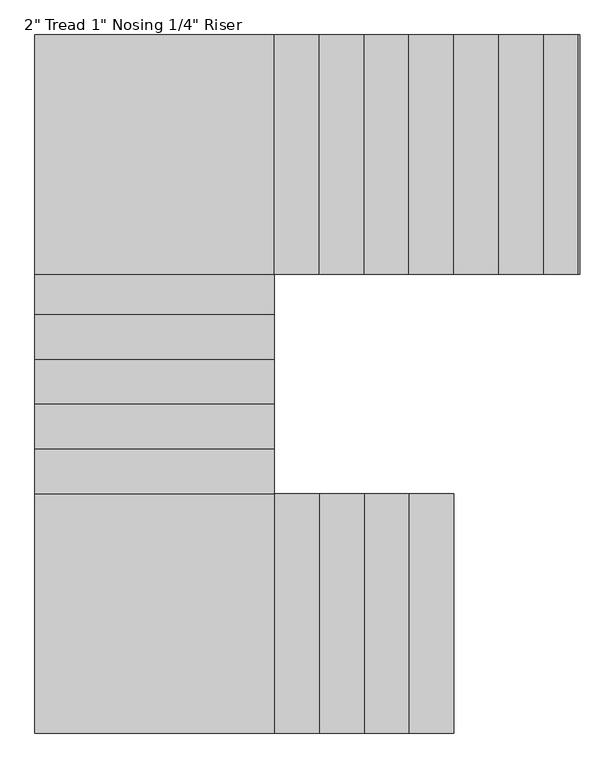
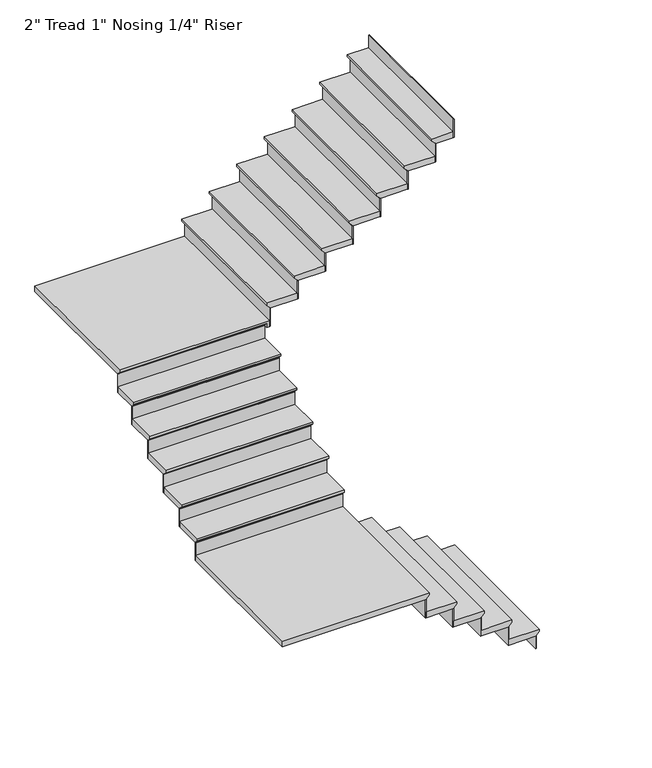
"""IFC4 building model written with IfcOpenShell, lengths in millimetres: stair flight geometry."""

from ifc_helpers import new_model, si_unit, origin, place, context, project, spatial, faceted_brep, source, transform, mapped, element, save


def stair_flight_0ad16ec4(model_context):
    return source(origin(), model_context, "Body", "Brep", [
        faceted_brep([(-2683.1105391, -1521.8373761, 141.3710526), (-2683.1105391, -1521.8373761, 160.4210526), (-2683.1105391, -2741.0373761, 160.4210526), (-2683.1105391, -2741.0373761, 141.3710526), (-2708.5105391, -1521.8373761, 115.9710526), (-2708.5105391, -2741.0373761, 115.9710526), (-2937.1105391, -1521.8373761, 160.4210526), (-2937.1105391, -2741.0373761, 160.4210526), (-2708.5105391, -2741.0373761, 109.6210526), (-2937.1105391, -2741.0373761, 109.6210526), (-2937.1105391, -1521.8373761, 109.6210526), (-2708.5105391, -1521.8373761, 109.6210526)], [[[0, 1, 2, 3]], [[4, 0, 3, 5]], [[2, 1, 6, 7]], [[8, 9, 10, 11]], [[2, 7, 9, 8, 5, 3]], [[8, 11, 4, 5]], [[6, 1, 0, 4, 11, 10]], [[7, 6, 10, 9]]]),
        faceted_brep([(-2708.5105391, -1521.8373761, 109.6210526), (-2708.5105391, -1521.8373761, 0.0), (-2714.8605391, -1521.8373761, 0.0), (-2714.8605391, -1521.8373761, 109.6210526), (-2708.5105391, -2741.0373761, 109.6210526), (-2714.8605391, -2741.0373761, 109.6210526), (-2714.8605391, -2741.0373761, 0.0), (-2708.5105391, -2741.0373761, 0.0)], [[[0, 1, 2, 3]], [[4, 5, 6, 7]], [[1, 0, 4, 7]], [[2, 1, 7, 6]], [[3, 2, 6, 5]], [[0, 3, 5, 4]]]),
        faceted_brep([(-2937.1105391, -1521.8373761, 270.0421053), (-2937.1105391, -1521.8373761, 109.6210526), (-2943.4605391, -1521.8373761, 109.6210526), (-2943.4605391, -1521.8373761, 270.0421053), (-2937.1105391, -2741.0373761, 270.0421053), (-2943.4605391, -2741.0373761, 270.0421053), (-2943.4605391, -2741.0373761, 109.6210526), (-2937.1105391, -2741.0373761, 109.6210526)], [[[0, 1, 2, 3]], [[4, 5, 6, 7]], [[1, 0, 4, 7]], [[2, 1, 7, 6]], [[3, 2, 6, 5]], [[0, 3, 5, 4]]]),
        faceted_brep([(-2911.7105391, -2741.0373761, 320.8421053), (-2911.7105391, -1521.8373761, 320.8421053), (-3165.7105391, -1521.8373761, 320.8421053), (-3165.7105391, -2741.0373761, 320.8421053), (-2937.1105391, -2741.0373761, 270.0421053), (-3165.7105391, -2741.0373761, 270.0421053), (-3165.7105391, -1521.8373761, 270.0421053), (-2937.1105391, -1521.8373761, 270.0421053), (-2937.1105391, -2741.0373761, 276.3921053), (-2911.7105391, -2741.0373761, 301.7921053), (-2937.1105391, -1521.8373761, 276.3921053), (-2911.7105391, -1521.8373761, 301.7921053)], [[[0, 1, 2, 3]], [[4, 5, 6, 7]], [[0, 3, 5, 4, 8, 9]], [[4, 7, 10, 8]], [[2, 1, 11, 10, 7, 6]], [[3, 2, 6, 5]], [[11, 1, 0, 9]], [[10, 11, 9, 8]]]),
        faceted_brep([(-3165.7105391, -1521.8373761, 430.4631579), (-3165.7105391, -1521.8373761, 270.0421053), (-3172.0605391, -1521.8373761, 270.0421053), (-3172.0605391, -1521.8373761, 430.4631579), (-3165.7105391, -2741.0373761, 430.4631579), (-3172.0605391, -2741.0373761, 430.4631579), (-3172.0605391, -2741.0373761, 270.0421053), (-3165.7105391, -2741.0373761, 270.0421053)], [[[0, 1, 2, 3]], [[4, 5, 6, 7]], [[1, 0, 4, 7]], [[2, 1, 7, 6]], [[3, 2, 6, 5]], [[0, 3, 5, 4]]]),
        faceted_brep([(-3140.3105391, -2741.0373761, 481.2631579), (-3140.3105391, -1521.8373761, 481.2631579), (-3394.3105391, -1521.8373761, 481.2631579), (-3394.3105391, -2741.0373761, 481.2631579), (-3165.7105391, -2741.0373761, 430.4631579), (-3394.3105391, -2741.0373761, 430.4631579), (-3394.3105391, -1521.8373761, 430.4631579), (-3165.7105391, -1521.8373761, 430.4631579), (-3165.7105391, -2741.0373761, 436.8131579), (-3140.3105391, -2741.0373761, 462.2131579), (-3165.7105391, -1521.8373761, 436.8131579), (-3140.3105391, -1521.8373761, 462.2131579)], [[[0, 1, 2, 3]], [[4, 5, 6, 7]], [[0, 3, 5, 4, 8, 9]], [[4, 7, 10, 8]], [[2, 1, 11, 10, 7, 6]], [[3, 2, 6, 5]], [[11, 1, 0, 9]], [[10, 11, 9, 8]]]),
        faceted_brep([(-3394.3105391, -1521.8373761, 590.8842105), (-3394.3105391, -1521.8373761, 430.4631579), (-3400.6605391, -1521.8373761, 430.4631579), (-3400.6605391, -1521.8373761, 590.8842105), (-3394.3105391, -2741.0373761, 590.8842105), (-3400.6605391, -2741.0373761, 590.8842105), (-3400.6605391, -2741.0373761, 430.4631579), (-3394.3105391, -2741.0373761, 430.4631579)], [[[0, 1, 2, 3]], [[4, 5, 6, 7]], [[1, 0, 4, 7]], [[2, 1, 7, 6]], [[3, 2, 6, 5]], [[0, 3, 5, 4]]]),
        faceted_brep([(-3368.9105391, -2741.0373761, 641.6842105), (-3368.9105391, -1521.8373761, 641.6842105), (-3622.9105391, -1521.8373761, 641.6842105), (-3622.9105391, -2741.0373761, 641.6842105), (-3394.3105391, -2741.0373761, 590.8842105), (-3622.9105391, -2741.0373761, 590.8842105), (-3622.9105391, -1521.8373761, 590.8842105), (-3394.3105391, -1521.8373761, 590.8842105), (-3394.3105391, -2741.0373761, 597.2342105), (-3368.9105391, -2741.0373761, 622.6342105), (-3394.3105391, -1521.8373761, 597.2342105), (-3368.9105391, -1521.8373761, 622.6342105)], [[[0, 1, 2, 3]], [[4, 5, 6, 7]], [[0, 3, 5, 4, 8, 9]], [[4, 7, 10, 8]], [[2, 1, 11, 10, 7, 6]], [[3, 2, 6, 5]], [[11, 1, 0, 9]], [[10, 11, 9, 8]]]),
        faceted_brep([(-3622.9105391, -1521.8373761, 751.3052632), (-3622.9105391, -1521.8373761, 590.8842105), (-3629.2605391, -1521.8373761, 590.8842105), (-3629.2605391, -1521.8373761, 751.3052632), (-3622.9105391, -2741.0373761, 751.3052632), (-3629.2605391, -2741.0373761, 751.3052632), (-3629.2605391, -2741.0373761, 590.8842105), (-3622.9105391, -2741.0373761, 590.8842105)], [[[0, 1, 2, 3]], [[4, 5, 6, 7]], [[1, 0, 4, 7]], [[2, 1, 7, 6]], [[3, 2, 6, 5]], [[0, 3, 5, 4]]]),
        faceted_brep([(-4816.7105391, -1496.4373761, 802.1052632), (-4816.7105391, -2741.0373761, 802.1052632), (-3597.5105391, -2741.0373761, 802.1052632), (-3597.5105391, -1496.4373761, 802.1052632), (-4816.7105391, -2741.0373761, 751.3052632), (-4816.7105391, -1496.4373761, 751.3052632), (-3597.5105391, -1496.4373761, 751.3052632), (-3597.5105391, -1521.8373761, 751.3052632), (-3622.9105391, -1521.8373761, 751.3052632), (-3622.9105391, -2741.0373761, 751.3052632), (-3622.9105391, -2741.0373761, 757.6552632), (-3597.5105391, -2741.0373761, 783.0552632), (-3622.9105391, -1521.8373761, 757.6552632), (-3597.5105391, -1521.8373761, 783.0552632)], [[[0, 1, 2, 3]], [[4, 5, 6, 7, 8, 9]], [[1, 0, 5, 4]], [[2, 1, 4, 9, 10, 11]], [[9, 8, 12, 10]], [[8, 7, 13, 12]], [[3, 2, 11, 13, 7, 6]], [[0, 3, 6, 5]], [[11, 10, 12, 13]]]),
        faceted_brep([(-3597.5105391, -1496.4373761, 911.7263158), (-3597.5105391, -1496.4373761, 751.3052632), (-3597.5105391, -1490.0873761, 751.3052632), (-3597.5105391, -1490.0873761, 911.7263158), (-4816.7105391, -1496.4373761, 911.7263158), (-4816.7105391, -1490.0873761, 911.7263158), (-4816.7105391, -1490.0873761, 751.3052632), (-4816.7105391, -1496.4373761, 751.3052632)], [[[0, 1, 2, 3]], [[4, 5, 6, 7]], [[1, 0, 4, 7]], [[2, 1, 7, 6]], [[3, 2, 6, 5]], [[0, 3, 5, 4]]]),
        faceted_brep([(-4816.7105391, -1521.8373761, 962.5263158), (-3597.5105391, -1521.8373761, 962.5263158), (-3597.5105391, -1267.8373761, 962.5263158), (-4816.7105391, -1267.8373761, 962.5263158), (-4816.7105391, -1496.4373761, 911.7263158), (-4816.7105391, -1267.8373761, 911.7263158), (-3597.5105391, -1267.8373761, 911.7263158), (-3597.5105391, -1496.4373761, 911.7263158), (-4816.7105391, -1496.4373761, 918.0763158), (-4816.7105391, -1521.8373761, 943.4763158), (-3597.5105391, -1496.4373761, 918.0763158), (-3597.5105391, -1521.8373761, 943.4763158)], [[[0, 1, 2, 3]], [[4, 5, 6, 7]], [[0, 3, 5, 4, 8, 9]], [[4, 7, 10, 8]], [[2, 1, 11, 10, 7, 6]], [[3, 2, 6, 5]], [[11, 1, 0, 9]], [[10, 11, 9, 8]]]),
        faceted_brep([(-3597.5105391, -1267.8373761, 1072.1473684), (-3597.5105391, -1267.8373761, 911.7263158), (-3597.5105391, -1261.4873761, 911.7263158), (-3597.5105391, -1261.4873761, 1072.1473684), (-4816.7105391, -1267.8373761, 1072.1473684), (-4816.7105391, -1261.4873761, 1072.1473684), (-4816.7105391, -1261.4873761, 911.7263158), (-4816.7105391, -1267.8373761, 911.7263158)], [[[0, 1, 2, 3]], [[4, 5, 6, 7]], [[1, 0, 4, 7]], [[2, 1, 7, 6]], [[3, 2, 6, 5]], [[0, 3, 5, 4]]]),
        faceted_brep([(-4816.7105391, -1293.2373761, 1122.9473684), (-3597.5105391, -1293.2373761, 1122.9473684), (-3597.5105391, -1039.2373761, 1122.9473684), (-4816.7105391, -1039.2373761, 1122.9473684), (-4816.7105391, -1267.8373761, 1072.1473684), (-4816.7105391, -1039.2373761, 1072.1473684), (-3597.5105391, -1039.2373761, 1072.1473684), (-3597.5105391, -1267.8373761, 1072.1473684), (-4816.7105391, -1267.8373761, 1078.4973684), (-4816.7105391, -1293.2373761, 1103.8973684), (-3597.5105391, -1267.8373761, 1078.4973684), (-3597.5105391, -1293.2373761, 1103.8973684)], [[[0, 1, 2, 3]], [[4, 5, 6, 7]], [[0, 3, 5, 4, 8, 9]], [[4, 7, 10, 8]], [[2, 1, 11, 10, 7, 6]], [[3, 2, 6, 5]], [[11, 1, 0, 9]], [[10, 11, 9, 8]]]),
        faceted_brep([(-3597.5105391, -1039.2373761, 1232.5684211), (-3597.5105391, -1039.2373761, 1072.1473684), (-3597.5105391, -1032.8873761, 1072.1473684), (-3597.5105391, -1032.8873761, 1232.5684211), (-4816.7105391, -1039.2373761, 1232.5684211), (-4816.7105391, -1032.8873761, 1232.5684211), (-4816.7105391, -1032.8873761, 1072.1473684), (-4816.7105391, -1039.2373761, 1072.1473684)], [[[0, 1, 2, 3]], [[4, 5, 6, 7]], [[1, 0, 4, 7]], [[2, 1, 7, 6]], [[3, 2, 6, 5]], [[0, 3, 5, 4]]]),
        faceted_brep([(-4816.7105391, -1064.6373761, 1283.3684211), (-3597.5105391, -1064.6373761, 1283.3684211), (-3597.5105391, -810.6373761, 1283.3684211), (-4816.7105391, -810.6373761, 1283.3684211), (-4816.7105391, -1039.2373761, 1232.5684211), (-4816.7105391, -810.6373761, 1232.5684211), (-3597.5105391, -810.6373761, 1232.5684211), (-3597.5105391, -1039.2373761, 1232.5684211), (-4816.7105391, -1039.2373761, 1238.9184211), (-4816.7105391, -1064.6373761, 1264.3184211), (-3597.5105391, -1039.2373761, 1238.9184211), (-3597.5105391, -1064.6373761, 1264.3184211)], [[[0, 1, 2, 3]], [[4, 5, 6, 7]], [[0, 3, 5, 4, 8, 9]], [[4, 7, 10, 8]], [[2, 1, 11, 10, 7, 6]], [[3, 2, 6, 5]], [[11, 1, 0, 9]], [[10, 11, 9, 8]]]),
        faceted_brep([(-3597.5105391, -810.6373761, 1392.9894737), (-3597.5105391, -810.6373761, 1232.5684211), (-3597.5105391, -804.2873761, 1232.5684211), (-3597.5105391, -804.2873761, 1392.9894737), (-4816.7105391, -810.6373761, 1392.9894737), (-4816.7105391, -804.2873761, 1392.9894737), (-4816.7105391, -804.2873761, 1232.5684211), (-4816.7105391, -810.6373761, 1232.5684211)], [[[0, 1, 2, 3]], [[4, 5, 6, 7]], [[1, 0, 4, 7]], [[2, 1, 7, 6]], [[3, 2, 6, 5]], [[0, 3, 5, 4]]]),
        faceted_brep([(-4816.7105391, -836.0373761, 1443.7894737), (-3597.5105391, -836.0373761, 1443.7894737), (-3597.5105391, -582.0373761, 1443.7894737), (-4816.7105391, -582.0373761, 1443.7894737), (-4816.7105391, -810.6373761, 1392.9894737), (-4816.7105391, -582.0373761, 1392.9894737), (-3597.5105391, -582.0373761, 1392.9894737), (-3597.5105391, -810.6373761, 1392.9894737), (-4816.7105391, -810.6373761, 1399.3394737), (-4816.7105391, -836.0373761, 1424.7394737), (-3597.5105391, -810.6373761, 1399.3394737), (-3597.5105391, -836.0373761, 1424.7394737)], [[[0, 1, 2, 3]], [[4, 5, 6, 7]], [[0, 3, 5, 4, 8, 9]], [[4, 7, 10, 8]], [[2, 1, 11, 10, 7, 6]], [[3, 2, 6, 5]], [[11, 1, 0, 9]], [[10, 11, 9, 8]]]),
        faceted_brep([(-3597.5105391, -582.0373761, 1553.4105263), (-3597.5105391, -582.0373761, 1392.9894737), (-3597.5105391, -575.6873761, 1392.9894737), (-3597.5105391, -575.6873761, 1553.4105263), (-4816.7105391, -582.0373761, 1553.4105263), (-4816.7105391, -575.6873761, 1553.4105263), (-4816.7105391, -575.6873761, 1392.9894737), (-4816.7105391, -582.0373761, 1392.9894737)], [[[0, 1, 2, 3]], [[4, 5, 6, 7]], [[1, 0, 4, 7]], [[2, 1, 7, 6]], [[3, 2, 6, 5]], [[0, 3, 5, 4]]]),
        faceted_brep([(-4816.7105391, -607.4373761, 1604.2105263), (-3597.5105391, -607.4373761, 1604.2105263), (-3597.5105391, -378.8373761, 1604.2105263), (-4816.7105391, -378.8373761, 1604.2105263), (-4816.7105391, -582.0373761, 1553.4105263), (-4816.7105391, -378.8373761, 1553.4105263), (-3597.5105391, -378.8373761, 1553.4105263), (-3597.5105391, -582.0373761, 1553.4105263), (-4816.7105391, -582.0373761, 1559.7605263), (-4816.7105391, -607.4373761, 1585.1605263), (-3597.5105391, -582.0373761, 1559.7605263), (-3597.5105391, -607.4373761, 1585.1605263)], [[[0, 1, 2, 3]], [[4, 5, 6, 7]], [[0, 3, 5, 4, 8, 9]], [[4, 7, 10, 8]], [[2, 1, 11, 10, 7, 6]], [[3, 2, 6, 5]], [[11, 1, 0, 9]], [[10, 11, 9, 8]]]),
        faceted_brep([(-3597.5105391, -378.8373761, 1713.8315789), (-3597.5105391, -378.8373761, 1553.4105263), (-3597.5105391, -372.4873761, 1553.4105263), (-3597.5105391, -372.4873761, 1713.8315789), (-4816.7105391, -378.8373761, 1713.8315789), (-4816.7105391, -372.4873761, 1713.8315789), (-4816.7105391, -372.4873761, 1553.4105263), (-4816.7105391, -378.8373761, 1553.4105263)], [[[0, 1, 2, 3]], [[4, 5, 6, 7]], [[1, 0, 4, 7]], [[2, 1, 7, 6]], [[3, 2, 6, 5]], [[0, 3, 5, 4]]]),
        faceted_brep([(-3572.1105391, 814.9626239, 1764.6315789), (-4816.7105391, 814.9626239, 1764.6315789), (-4816.7105391, -404.2373761, 1764.6315789), (-3572.1105391, -404.2373761, 1764.6315789), (-4816.7105391, 814.9626239, 1713.8315789), (-3572.1105391, 814.9626239, 1713.8315789), (-3572.1105391, -404.2373761, 1713.8315789), (-3597.5105391, -404.2373761, 1713.8315789), (-3597.5105391, -378.8373761, 1713.8315789), (-4816.7105391, -378.8373761, 1713.8315789), (-4816.7105391, -378.8373761, 1720.1815789), (-4816.7105391, -404.2373761, 1745.5815789), (-3597.5105391, -378.8373761, 1720.1815789), (-3597.5105391, -404.2373761, 1745.5815789)], [[[0, 1, 2, 3]], [[4, 5, 6, 7, 8, 9]], [[1, 0, 5, 4]], [[2, 1, 4, 9, 10, 11]], [[9, 8, 12, 10]], [[8, 7, 13, 12]], [[3, 2, 11, 13, 7, 6]], [[0, 3, 6, 5]], [[11, 10, 12, 13]]]),
        faceted_brep([(-3572.1105391, -404.2373761, 1874.2526316), (-3572.1105391, -404.2373761, 1713.8315789), (-3565.7605391, -404.2373761, 1713.8315789), (-3565.7605391, -404.2373761, 1874.2526316), (-3572.1105391, 814.9626239, 1874.2526316), (-3565.7605391, 814.9626239, 1874.2526316), (-3565.7605391, 814.9626239, 1713.8315789), (-3572.1105391, 814.9626239, 1713.8315789)], [[[0, 1, 2, 3]], [[4, 5, 6, 7]], [[1, 0, 4, 7]], [[2, 1, 7, 6]], [[3, 2, 6, 5]], [[0, 3, 5, 4]]]),
        faceted_brep([(-3597.5105391, 814.9626239, 1925.0526316), (-3597.5105391, -404.2373761, 1925.0526316), (-3343.5105391, -404.2373761, 1925.0526316), (-3343.5105391, 814.9626239, 1925.0526316), (-3572.1105391, 814.9626239, 1874.2526316), (-3343.5105391, 814.9626239, 1874.2526316), (-3343.5105391, -404.2373761, 1874.2526316), (-3572.1105391, -404.2373761, 1874.2526316), (-3572.1105391, 814.9626239, 1880.6026316), (-3597.5105391, 814.9626239, 1906.0026316), (-3572.1105391, -404.2373761, 1880.6026316), (-3597.5105391, -404.2373761, 1906.0026316)], [[[0, 1, 2, 3]], [[4, 5, 6, 7]], [[0, 3, 5, 4, 8, 9]], [[4, 7, 10, 8]], [[2, 1, 11, 10, 7, 6]], [[3, 2, 6, 5]], [[11, 1, 0, 9]], [[10, 11, 9, 8]]]),
        faceted_brep([(-3343.5105391, -404.2373761, 2034.6736842), (-3343.5105391, -404.2373761, 1874.2526316), (-3337.1605391, -404.2373761, 1874.2526316), (-3337.1605391, -404.2373761, 2034.6736842), (-3343.5105391, 814.9626239, 2034.6736842), (-3337.1605391, 814.9626239, 2034.6736842), (-3337.1605391, 814.9626239, 1874.2526316), (-3343.5105391, 814.9626239, 1874.2526316)], [[[0, 1, 2, 3]], [[4, 5, 6, 7]], [[1, 0, 4, 7]], [[2, 1, 7, 6]], [[3, 2, 6, 5]], [[0, 3, 5, 4]]]),
        faceted_brep([(-3368.9105391, 814.9626239, 2085.4736842), (-3368.9105391, -404.2373761, 2085.4736842), (-3114.9105391, -404.2373761, 2085.4736842), (-3114.9105391, 814.9626239, 2085.4736842), (-3343.5105391, 814.9626239, 2034.6736842), (-3114.9105391, 814.9626239, 2034.6736842), (-3114.9105391, -404.2373761, 2034.6736842), (-3343.5105391, -404.2373761, 2034.6736842), (-3343.5105391, 814.9626239, 2041.0236842), (-3368.9105391, 814.9626239, 2066.4236842), (-3343.5105391, -404.2373761, 2041.0236842), (-3368.9105391, -404.2373761, 2066.4236842)], [[[0, 1, 2, 3]], [[4, 5, 6, 7]], [[0, 3, 5, 4, 8, 9]], [[4, 7, 10, 8]], [[2, 1, 11, 10, 7, 6]], [[3, 2, 6, 5]], [[11, 1, 0, 9]], [[10, 11, 9, 8]]]),
        faceted_brep([(-3114.9105391, -404.2373761, 2195.0947368), (-3114.9105391, -404.2373761, 2034.6736842), (-3108.5605391, -404.2373761, 2034.6736842), (-3108.5605391, -404.2373761, 2195.0947368), (-3114.9105391, 814.9626239, 2195.0947368), (-3108.5605391, 814.9626239, 2195.0947368), (-3108.5605391, 814.9626239, 2034.6736842), (-3114.9105391, 814.9626239, 2034.6736842)], [[[0, 1, 2, 3]], [[4, 5, 6, 7]], [[1, 0, 4, 7]], [[2, 1, 7, 6]], [[3, 2, 6, 5]], [[0, 3, 5, 4]]]),
        faceted_brep([(-3140.3105391, 814.9626239, 2245.8947368), (-3140.3105391, -404.2373761, 2245.8947368), (-2886.3105391, -404.2373761, 2245.8947368), (-2886.3105391, 814.9626239, 2245.8947368), (-3114.9105391, 814.9626239, 2195.0947368), (-2886.3105391, 814.9626239, 2195.0947368), (-2886.3105391, -404.2373761, 2195.0947368), (-3114.9105391, -404.2373761, 2195.0947368), (-3114.9105391, 814.9626239, 2201.4447368), (-3140.3105391, 814.9626239, 2226.8447368), (-3114.9105391, -404.2373761, 2201.4447368), (-3140.3105391, -404.2373761, 2226.8447368)], [[[0, 1, 2, 3]], [[4, 5, 6, 7]], [[0, 3, 5, 4, 8, 9]], [[4, 7, 10, 8]], [[2, 1, 11, 10, 7, 6]], [[3, 2, 6, 5]], [[11, 1, 0, 9]], [[10, 11, 9, 8]]]),
        faceted_brep([(-2886.3105391, -404.2373761, 2355.5157895), (-2886.3105391, -404.2373761, 2195.0947368), (-2879.9605391, -404.2373761, 2195.0947368), (-2879.9605391, -404.2373761, 2355.5157895), (-2886.3105391, 814.9626239, 2355.5157895), (-2879.9605391, 814.9626239, 2355.5157895), (-2879.9605391, 814.9626239, 2195.0947368), (-2886.3105391, 814.9626239, 2195.0947368)], [[[0, 1, 2, 3]], [[4, 5, 6, 7]], [[1, 0, 4, 7]], [[2, 1, 7, 6]], [[3, 2, 6, 5]], [[0, 3, 5, 4]]]),
        faceted_brep([(-2911.7105391, 814.9626239, 2406.3157895), (-2911.7105391, -404.2373761, 2406.3157895), (-2657.7105391, -404.2373761, 2406.3157895), (-2657.7105391, 814.9626239, 2406.3157895), (-2886.3105391, 814.9626239, 2355.5157895), (-2657.7105391, 814.9626239, 2355.5157895), (-2657.7105391, -404.2373761, 2355.5157895), (-2886.3105391, -404.2373761, 2355.5157895), (-2886.3105391, 814.9626239, 2361.8657895), (-2911.7105391, 814.9626239, 2387.2657895), (-2886.3105391, -404.2373761, 2361.8657895), (-2911.7105391, -404.2373761, 2387.2657895)], [[[0, 1, 2, 3]], [[4, 5, 6, 7]], [[0, 3, 5, 4, 8, 9]], [[4, 7, 10, 8]], [[2, 1, 11, 10, 7, 6]], [[3, 2, 6, 5]], [[11, 1, 0, 9]], [[10, 11, 9, 8]]]),
        faceted_brep([(-2657.7105391, -404.2373761, 2515.9368421), (-2657.7105391, -404.2373761, 2355.5157895), (-2651.3605391, -404.2373761, 2355.5157895), (-2651.3605391, -404.2373761, 2515.9368421), (-2657.7105391, 814.9626239, 2515.9368421), (-2651.3605391, 814.9626239, 2515.9368421), (-2651.3605391, 814.9626239, 2355.5157895), (-2657.7105391, 814.9626239, 2355.5157895)], [[[0, 1, 2, 3]], [[4, 5, 6, 7]], [[1, 0, 4, 7]], [[2, 1, 7, 6]], [[3, 2, 6, 5]], [[0, 3, 5, 4]]]),
        faceted_brep([(-2683.1105391, 814.9626239, 2566.7368421), (-2683.1105391, -404.2373761, 2566.7368421), (-2429.1105391, -404.2373761, 2566.7368421), (-2429.1105391, 814.9626239, 2566.7368421), (-2657.7105391, 814.9626239, 2515.9368421), (-2429.1105391, 814.9626239, 2515.9368421), (-2429.1105391, -404.2373761, 2515.9368421), (-2657.7105391, -404.2373761, 2515.9368421), (-2657.7105391, 814.9626239, 2522.2868421), (-2683.1105391, 814.9626239, 2547.6868421), (-2657.7105391, -404.2373761, 2522.2868421), (-2683.1105391, -404.2373761, 2547.6868421)], [[[0, 1, 2, 3]], [[4, 5, 6, 7]], [[0, 3, 5, 4, 8, 9]], [[4, 7, 10, 8]], [[2, 1, 11, 10, 7, 6]], [[3, 2, 6, 5]], [[11, 1, 0, 9]], [[10, 11, 9, 8]]]),
        faceted_brep([(-2429.1105391, -404.2373761, 2676.3578947), (-2429.1105391, -404.2373761, 2515.9368421), (-2422.7605391, -404.2373761, 2515.9368421), (-2422.7605391, -404.2373761, 2676.3578947), (-2429.1105391, 814.9626239, 2676.3578947), (-2422.7605391, 814.9626239, 2676.3578947), (-2422.7605391, 814.9626239, 2515.9368421), (-2429.1105391, 814.9626239, 2515.9368421)], [[[0, 1, 2, 3]], [[4, 5, 6, 7]], [[1, 0, 4, 7]], [[2, 1, 7, 6]], [[3, 2, 6, 5]], [[0, 3, 5, 4]]]),
        faceted_brep([(-2454.5105391, 814.9626239, 2727.1578947), (-2454.5105391, -404.2373761, 2727.1578947), (-2200.5105391, -404.2373761, 2727.1578947), (-2200.5105391, 814.9626239, 2727.1578947), (-2429.1105391, 814.9626239, 2676.3578947), (-2200.5105391, 814.9626239, 2676.3578947), (-2200.5105391, -404.2373761, 2676.3578947), (-2429.1105391, -404.2373761, 2676.3578947), (-2429.1105391, 814.9626239, 2682.7078947), (-2454.5105391, 814.9626239, 2708.1078947), (-2429.1105391, -404.2373761, 2682.7078947), (-2454.5105391, -404.2373761, 2708.1078947)], [[[0, 1, 2, 3]], [[4, 5, 6, 7]], [[0, 3, 5, 4, 8, 9]], [[4, 7, 10, 8]], [[2, 1, 11, 10, 7, 6]], [[3, 2, 6, 5]], [[11, 1, 0, 9]], [[10, 11, 9, 8]]]),
        faceted_brep([(-2200.5105391, -404.2373761, 2836.7789474), (-2200.5105391, -404.2373761, 2676.3578947), (-2194.1605391, -404.2373761, 2676.3578947), (-2194.1605391, -404.2373761, 2836.7789474), (-2200.5105391, 814.9626239, 2836.7789474), (-2194.1605391, 814.9626239, 2836.7789474), (-2194.1605391, 814.9626239, 2676.3578947), (-2200.5105391, 814.9626239, 2676.3578947)], [[[0, 1, 2, 3]], [[4, 5, 6, 7]], [[1, 0, 4, 7]], [[2, 1, 7, 6]], [[3, 2, 6, 5]], [[0, 3, 5, 4]]]),
        faceted_brep([(-2048.1105391, -404.2373761, 2997.2), (-2048.1105391, -404.2373761, 2836.7789474), (-2041.7605391, -404.2373761, 2836.7789474), (-2041.7605391, -404.2373761, 2997.2), (-2048.1105391, 814.9626239, 2997.2), (-2041.7605391, 814.9626239, 2997.2), (-2041.7605391, 814.9626239, 2836.7789474), (-2048.1105391, 814.9626239, 2836.7789474)], [[[0, 1, 2, 3]], [[4, 5, 6, 7]], [[1, 0, 4, 7]], [[2, 1, 7, 6]], [[3, 2, 6, 5]], [[0, 3, 5, 4]]]),
        faceted_brep([(-2225.9105391, 814.9626239, 2887.5789474), (-2225.9105391, -404.2373761, 2887.5789474), (-2048.1105391, -404.2373761, 2887.5789474), (-2048.1105391, 814.9626239, 2887.5789474), (-2200.5105391, 814.9626239, 2836.7789474), (-2048.1105391, 814.9626239, 2836.7789474), (-2048.1105391, -404.2373761, 2836.7789474), (-2200.5105391, -404.2373761, 2836.7789474), (-2200.5105391, 814.9626239, 2843.1289474), (-2225.9105391, 814.9626239, 2868.5289474), (-2200.5105391, -404.2373761, 2843.1289474), (-2225.9105391, -404.2373761, 2868.5289474)], [[[0, 1, 2, 3]], [[4, 5, 6, 7]], [[0, 3, 5, 4, 8, 9]], [[4, 7, 10, 8]], [[2, 1, 11, 10, 7, 6]], [[3, 2, 6, 5]], [[11, 1, 0, 9]], [[10, 11, 9, 8]]]),
    ])


if __name__ == "__main__":
    model = new_model("IFC4")
    model_context = context("Model", 3, world=origin())
    ifc_project = project(units=[si_unit("LENGTHUNIT", "METRE", prefix="MILLI")], contexts=[model_context])
    site = spatial("IfcSite", under=ifc_project)
    building = spatial("IfcBuilding", under=site)
    placement = place(None, origin())
    stair_flight_shape = stair_flight_0ad16ec4(model_context)
    element("IfcStairFlight", 1, ObjectType="2\" Tread 1\" Nosing 1/4\" Riser", at=placement, inside=building, context=model_context, shape_type="MappedRepresentation", body=[
        mapped(stair_flight_shape, transform((0.0, 0.0, 0.0), x_axis=(1.0, 0.0, 0.0), y_axis=(0.0, 1.0, 0.0), z_axis=(0.0, 0.0, 1.0))),
    ])
    save(model, "model.ifc")
